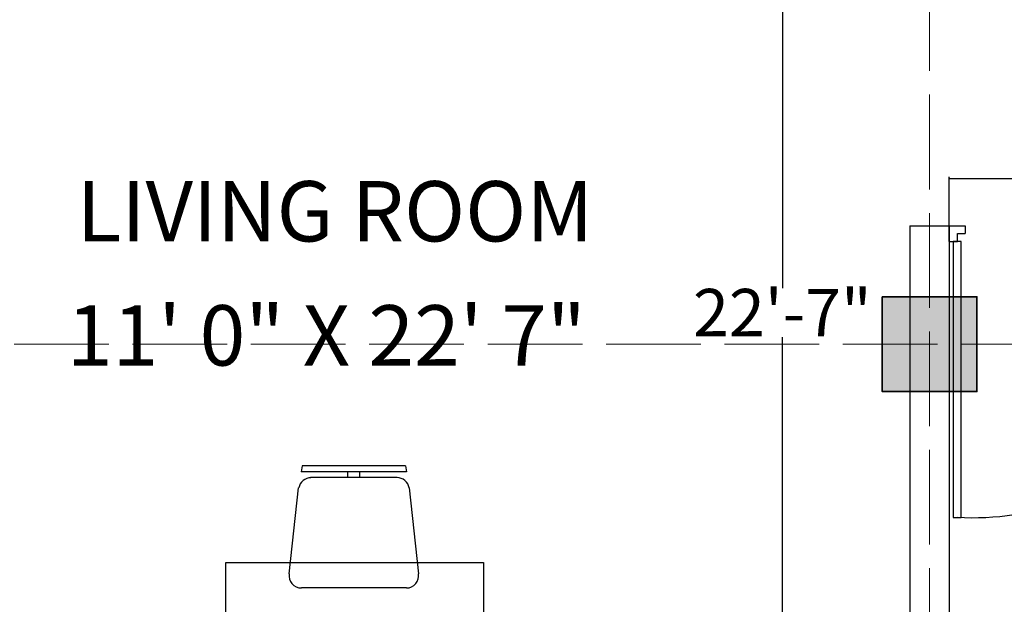
# Model space of a CAD drawing. Units: inches. Extents: x -113 to 5399, y -1393 to 3302.
# Tile 33 of 40: x 3405 to 3530, y 2688 to 2762. Entities that reach past the tile are written whole.
import ezdxf

# ---------------------------------------------------------------- set-up
doc = ezdxf.new("R2010")
doc.units = ezdxf.units.IN
doc.header["$MEASUREMENT"] = 0
doc.linetypes.add('ACAD_ISO02W100', pattern=[15, 12, -3])
for name, color, linetype, lineweight in [('A-ANNO-DIMS', 254, 'Continuous', 18), ('A-AREA-IDEN', 4, 'Continuous', 18), ('A-COLS', 7, 'Continuous', 35), ('doors', 2, 'Continuous', 25), ('furniture', 131, 'Continuous', 18), ('GRIDS', 7, 'ACAD_ISO02W100', 13), ('walls', 1, 'Continuous', 25)]:
    doc.layers.add(name, color=color, linetype=linetype, lineweight=lineweight)
doc.layers.add('B-FURNITURE', color=22, linetype='Continuous')
doc.styles.get("Standard").update_dxf_attribs({"font": 'arial.ttf'})
doc.dimstyles.get("Standard").update_dxf_attribs({"dimtxt": 6, "dimasz": 0.18, "dimexe": 0.18, "dimexo": 0.0625, "dimgap": 0.09, "dimtad": 0, "dimtih": 1, "dimtoh": 1, "dimdec": 1, "dimzin": 0, "dimdsep": 46, "dimlunit": 4, "dimtxsty": 'Standard', "dimblk": 'ARCHTICK', "dimcen": 0.09, "dimadec": 0, "dimazin": 0, "dimtfac": 1, "dimtdec": 1, "dimtofl": 0, "dimtmove": 0, "dimatfit": 3, "dimfxl": 1, "dimtolj": 1, "dimtzin": 0, "dimarcsym": 0})

# ---------------------------------------------------------------- blocks, each defined once
blk = doc.blocks.new('A$C6ACA79D1')
at = {"layer": 'B-FURNITURE'}
for p, q in [((-0.5034, 0.0535), (-0.8012, -0.2442)), ((-0.5034, 0.0535), (-0.4835, 0.0392)), ((0.7869, -0.259), (0.4835, 0.0444)), ((0.4842, 0.0434), (0.5041, 0.0577)), ((0.8012, -0.239), (0.5034, 0.0587)), ((-0.4835, 0.0392), (-0.7869, -0.2642)), ((-0.4291, 0.0003), (-0.1547, -0.2204)), ((0.7427, -0.249), (0.4935, 0.0002)), ((-0.4935, -0.005), (-0.7427, -0.2542)), ((-0.601, -0.1125), (-0.6181, -0.0954)), ((0.601, -0.1073), (0.6181, -0.0902)), ((-0.6352, -0.1467), (-0.6523, -0.1296)), ((0.6352, -0.1415), (0.6523, -0.1244)), ((0.8012, -0.239), (0.7869, -0.259)), ((-0.7859, -0.2635), (-0.8002, -0.2436)), ((-0.1485, -0.2964), (-0.4513, -0.5992)), ((0.4513, -0.594), (0.1485, -0.2912)), ((0.748, -0.3133), (0.5273, -0.5877)), ((-0.1485, -1.1937), (-0.4513, -0.8909)), ((0.4513, -0.8961), (0.1485, -1.199)), ((0.748, -1.1768), (0.5273, -0.9024)), ((-0.7859, -1.2266), (-0.8002, -1.2466)), ((-0.4835, -1.5293), (-0.7869, -1.226)), ((-0.4935, -1.4851), (-0.7427, -1.236)), ((0.7869, -1.2312), (0.4835, -1.5346)), ((0.7427, -1.2412), (0.4935, -1.4903)), ((0.8012, -1.2511), (0.7869, -1.2312)), ((-0.5034, -1.5436), (-0.8012, -1.2459)), ((-0.4291, -1.4904), (-0.1547, -1.2698)), ((0.8012, -1.2511), (0.5034, -1.5488)), ((-0.6352, -1.3434), (-0.6523, -1.3605)), ((0.6352, -1.3486), (0.6523, -1.3657)), ((-0.601, -1.3776), (-0.6181, -1.3948)), ((0.601, -1.3829), (0.6181, -1.4)), ((-0.5034, -1.5436), (-0.4835, -1.5293)), ((0.4842, -1.5336), (0.5041, -1.5478))]:
    blk.add_line(p, q, dxfattribs=at)
at = {"layer": 'B-FURNITURE', "ltscale": 300}
for p, q in [((0.1547, -0.2152), (0.4291, 0.0055)), ((-0.5273, -0.593), (-0.748, -0.3186)), ((-0.5273, -0.8972), (-0.748, -1.1716)), ((0.1547, -1.275), (0.4291, -1.4956))]:
    blk.add_line(p, q, dxfattribs=at)
blk.add_lwpolyline([(-0.7425, -0.7425), (0, 0), (0.7425, -0.7425), (0, -1.4849)], close=True, dxfattribs=at)
at = {"layer": 'B-FURNITURE', "ltscale": 400}
for centre, start, end in [((-0.4582, -0.0403), 54.4069, 135), ((0.4589, -0.0361), 45, 125.5931), ((-0.7063, -0.2888), 135, 215.5931), ((0.7073, -0.2843), 324.4069, 45), ((-0.7063, -1.2013), 144.4069, 225), ((0.7073, -1.2059), 315, 35.5931), ((-0.4582, -1.4498), 225, 305.5931), ((0.4589, -1.454), 234.4069, 315)]:
    blk.add_arc(centre, 0.0499, start, end, dxfattribs=at)
at = {"layer": 'B-FURNITURE', "ltscale": 300}
for centre, start, end in [((-0.1838, -0.261), 315, 54.4069), ((0.1838, -0.2558), 125.5931, 225), ((-0.4866, -0.5639), 215.5931, 315), ((0.4866, -0.5586), 225, 324.4069), ((-0.4866, -0.9263), 45, 144.4069), ((0.4866, -0.9315), 35.5931, 135), ((-0.1838, -1.2291), 305.5931, 45), ((0.1838, -1.2343), 135, 234.4069)]:
    blk.add_arc(centre, 0.05, start, end, dxfattribs=at)
blk = doc.blocks.new('_ArchTick')
at = {"color": 0, "linetype": 'ByBlock', "const_width": 0.15}
blk.add_lwpolyline([(-0.5, -0.5), (0.5, 0.5)], dxfattribs=at)
blk = doc.blocks.new('*D127')
at = {"layer": 'A-ANNO-DIMS', "color": 0, "lineweight": -2, "transparency": 16777216}
for p, q in [((3501.73, 2860.06), (3501.22, 2860.06)), ((3501.4, 2860.06), (3501.4, 2727.66)), ((3501.4, 2589.06), (3501.4, 2721.46)), ((3501.73, 2589.06), (3501.22, 2589.06))]:
    blk.add_line(p, q, dxfattribs=at)
at = {"layer": 'Defpoints', "color": 0, "transparency": 16777216}
for p in [(3501.8, 2860.06), (3501.4, 2589.06), (3501.8, 2589.06)]:
    blk.add_point(p, dxfattribs=at)
at = {"layer": 'A-ANNO-DIMS', "color": 0, "lineweight": -2, "transparency": 16777216, "xscale": 0.18, "yscale": 0.18, "zscale": 0.18}
for p, rotation in [((3501.4, 2860.06), 90), ((3501.4, 2589.06), 270)]:
    blk.add_blockref('_ArchTick', p, dxfattribs=dict(at, rotation=rotation))
at = {"layer": 'A-ANNO-DIMS', "color": 0, "transparency": 16777216, "insert": (3501.4, 2724.56), "char_height": 6, "attachment_point": 5}
blk.add_mtext('\\A1;22\'-7"', dxfattribs=at)
blk = doc.blocks.new('COLUMN-12IN-SQUARE')
h = blk.add_hatch(color=256)
h.dxf.hatch_style = 1
h.paths.add_polyline_path([(6, 6), (-6, 6), (-6, -6), (6, -6)])
blk.add_lwpolyline([(-6, 6), (6, 6), (6, -6), (-6, -6)], close=True)
blk = doc.blocks.new('DOOR-SINGLE-36IN-PLAN')
for p, q in [((0.5, 2), (0.5, 36.98)), ((0.5, 36.98), (1.5, 36.98)), ((1.5, 36.98), (1.5, 2)), ((0, 2), (0, 0)), ((0, 2), (1.04, 2)), ((1.5, 2), (0.5, 2)), ((1.04, 2), (1.04, 0.98)), ((40, 2), (38.96, 2)), ((38.96, 2), (38.96, 0.98)), ((40, 0), (40, 2)), ((1.04, 0.98), (2, 0.98)), ((2, 0), (2, 0.98)), ((38.96, 0.98), (38, 0.98)), ((38, 0), (38, 0.98)), ((0, 0), (2, 0)), ((0, 0), (2, 0)), ((38, 0), (40, 0))]:
    blk.add_line(p, q)
blk.add_arc((2.94, 0.99), 36.04, 1.6003, 93.0893)
blk = doc.blocks.new('*D175')
at = {"layer": 'A-ANNO-DIMS', "color": 0, "lineweight": -2, "transparency": 16777216}
for p, q in [((3522.55, 2735.62), (3522.55, 2741.74)), ((3562.55, 2735.62), (3562.55, 2741.74)), ((3522.55, 2741.56), (3562.55, 2741.56)), ((3562.55, 2741.56), (3562.73, 2741.56))]:
    blk.add_line(p, q, dxfattribs=at)
at = {"layer": 'Defpoints', "color": 0, "transparency": 16777216}
for p in [(3562.55, 2741.56), (3522.55, 2735.56), (3562.55, 2735.56)]:
    blk.add_point(p, dxfattribs=at)
at = {"layer": 'A-ANNO-DIMS', "color": 0, "lineweight": -2, "transparency": 16777216, "xscale": 0.18, "yscale": 0.18, "zscale": 0.18, "rotation": 180}
blk.add_blockref('_ArchTick', (3522.55, 2741.56), dxfattribs=at)
at = {"layer": 'A-ANNO-DIMS', "color": 0, "lineweight": -2, "transparency": 16777216, "xscale": 0.18, "yscale": 0.18, "zscale": 0.18}
blk.add_blockref('_ArchTick', (3562.55, 2741.56), dxfattribs=at)
at = {"layer": 'A-ANNO-DIMS', "color": 0, "transparency": 16777216, "insert": (3610.19, 2741.56), "char_height": 6, "attachment_point": 5}
blk.add_mtext('\\A1;SWING DOOR 3\'-4" TYP.', dxfattribs=at)

msp = doc.modelspace()

# ---------------------------------------------------------------- linework, layer by layer
at = {"layer": 'GRIDS'}
for p, q in [((3520.05, 3262.17), (3520.05, 2490.34)), ((3104.07, 2720.56), (3762.86, 2720.56))]:
    msp.add_line(p, q, dxfattribs=at)
at = {"layer": 'walls'}
for p, q in [((3517.55, 2735.56), (3517.55, 2661.06)), ((3517.55, 2735.56), (3522.55, 2735.56)), ((3522.55, 2735.56), (3522.55, 2589.06))]:
    msp.add_line(p, q, dxfattribs=at)

# ---------------------------------------------------------------- block references
at = {"layer": 'A-COLS'}
msp.add_blockref('COLUMN-12IN-SQUARE', (3520.05, 2720.56), dxfattribs=at)
at = {"layer": 'doors', "extrusion": (0, 0, -1), "zscale": -1, "rotation": 180}
msp.add_blockref('DOOR-SINGLE-36IN-PLAN', (-3522.55, 2735.56), dxfattribs=at)
at = {"layer": 'furniture', "xscale": 31.0665876167328, "yscale": 31.0665876167328, "zscale": 31.0665876167328, "rotation": 314.9999999999397}
msp.add_blockref('A$C6ACA79D1', (3463.54, 2692.92), dxfattribs=at)

# ---------------------------------------------------------------- texts
at = {"layer": 'A-AREA-IDEN'}
for s, p in [('LIVING ROOM', (3412.01, 2733.57)), ('11\' 0" X 22\' 7"', (3410.76, 2717.85))]:
    msp.add_text(s, height=7.6473, dxfattribs=at).set_placement(p)

# ---------------------------------------------------------------- dimensions: what is measured, and where the dimension line sits
at = {"layer": 'A-ANNO-DIMS'}
dim = msp.add_linear_dim(base=(3501.4, 2589.06), p1=(3501.8, 2860.06), p2=(3501.8, 2589.06), angle=90, dimstyle='Standard', override={"dimclrd": 0, "dimclre": 0, "dimclrt": 0}, dxfattribs=at)
dim.commit()
dim.dimension.update_dxf_attribs({"geometry": '*D127', "text_midpoint": (3501.4, 2724.56)})
dim = msp.add_linear_dim(base=(3562.55, 2741.56), p1=(3522.55, 2735.56), p2=(3562.55, 2735.56), text='SWING DOOR <> TYP.', dimstyle='Standard', override={"dimdec": 1, "dimlfac": 1, "dimrnd": 0, "dimzin": 1, "dimdsep": 46, "dimlunit": 4, "dimfrac": 2}, dxfattribs=at)
dim.commit()
dim.dimension.update_dxf_attribs({"geometry": '*D175', "text_midpoint": (3610.19, 2741.56)})

doc.saveas('drawing.dxf')
